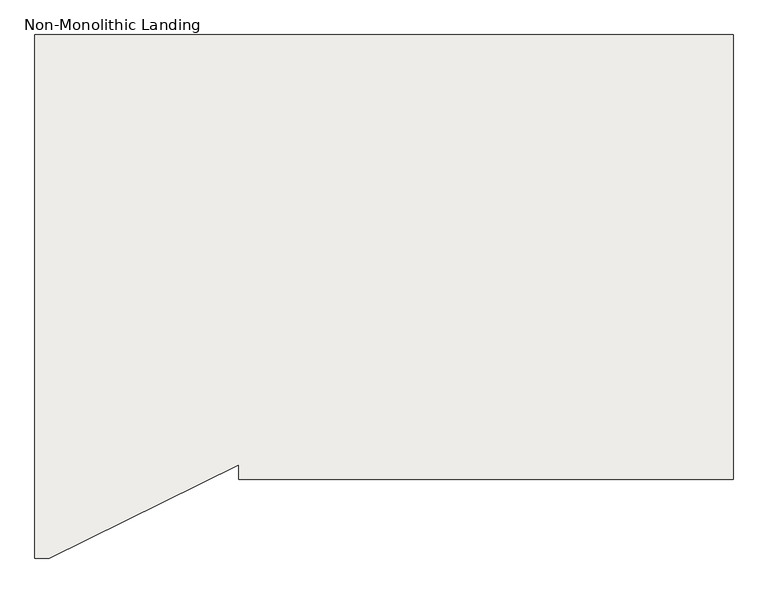
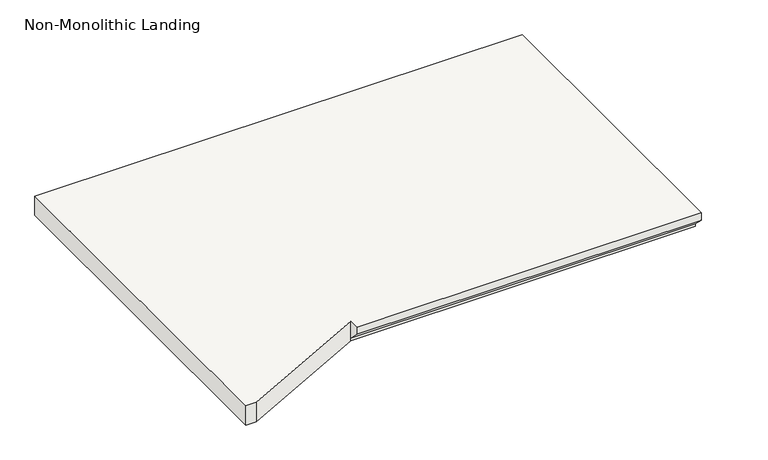
"""IFC4 building model written with IfcOpenShell, lengths in millimetres: slab geometry, Non-Monolithic Landing."""

from ifc_helpers import new_model, si_unit, origin, place, context, project, spatial, faceted_brep, source, transform, mapped, element, save


def non_monolithic_landing_e53bceee(model_context):
    return source(origin(), model_context, "Body", "Brep", [
        faceted_brep([(-2063.8102521, 6147.09939, 1843.6166667), (-2063.8102521, 6147.09939, 1862.6666667), (-2063.8102521, 6172.49939, 1862.6666667), (-2063.8102521, 6172.49939, 1818.2166667), (-1200.9932736, 6147.09939, 1843.6166667), (-1200.9932736, 6147.09939, 1862.6666667), (-1200.9932736, 6172.49939, 1818.2166667), (-1200.9932736, 6923.9200123, 1862.6666667), (-2394.7932736, 6923.9200123, 1862.6666667), (-2420.1932736, 6923.9200123, 1862.6666667), (-2420.1932736, 6009.5200123, 1862.6666667), (-2394.7932736, 6009.5200123, 1862.6666667), (-1200.9932736, 6172.49939, 1811.8666667), (-2063.8102521, 6172.49939, 1811.8666667), (-2394.7932736, 6009.5200123, 1811.8666667), (-2420.1932736, 6009.5200123, 1811.8666667), (-2420.1932736, 6923.9200123, 1811.8666667), (-2394.7932736, 6923.9200123, 1811.8666667), (-1200.9932736, 6923.9200123, 1811.8666667)], [[[0, 1, 2, 3]], [[4, 5, 1, 0]], [[6, 4, 0, 3]], [[7, 8, 9, 10, 11, 2, 1, 5]], [[12, 13, 14, 15, 16, 17, 18]], [[13, 12, 6, 3]], [[7, 5, 4, 6, 12, 18]], [[8, 7, 18, 17]], [[9, 8, 17, 16]], [[10, 9, 16, 15]], [[11, 10, 15, 14]], [[2, 11, 14, 13, 3]]]),
    ])


if __name__ == "__main__":
    model = new_model("IFC4")
    model_context = context("Model", 3, world=origin())
    ifc_project = project(units=[si_unit("LENGTHUNIT", "METRE", prefix="MILLI")], contexts=[model_context])
    site = spatial("IfcSite", under=ifc_project)
    building = spatial("IfcBuilding", under=site)
    placement = place(None, origin())
    non_monolithic_landing_shape = non_monolithic_landing_e53bceee(model_context)
    element("IfcSlab", 1, ObjectType="Non-Monolithic Landing", at=placement, inside=building, context=model_context, shape_type="MappedRepresentation", body=[
        mapped(non_monolithic_landing_shape, transform((0.0, 0.0, 0.0), x_axis=(1.0, 0.0, 0.0), y_axis=(0.0, 1.0, 0.0), z_axis=(0.0, 0.0, 1.0))),
    ])
    save(model, "model.ifc")
